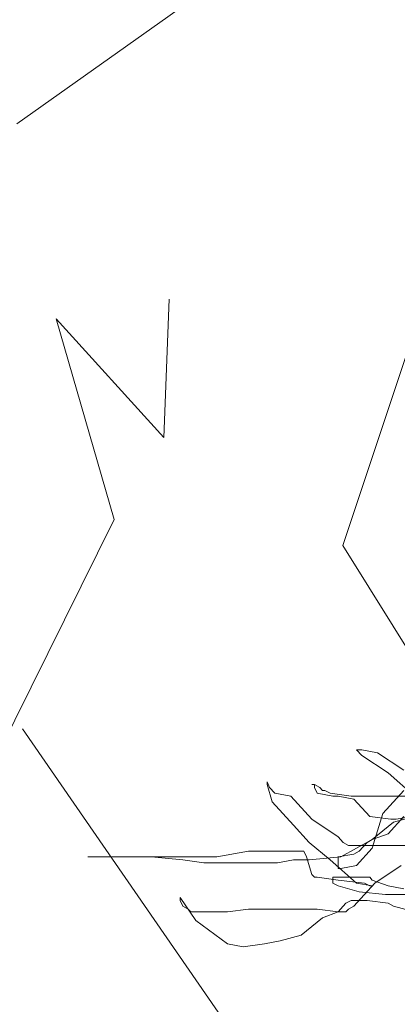
# Model space of a CAD drawing. Units: inches. Extents: x 1994 to 3075, y 3517 to 3950.
# Tile 37 of 58: x 1994.63804 to 1994.64257, y 3553.7375 to 3553.74931. Entities that reach past the tile are written whole.
import ezdxf

# ---------------------------------------------------------------- set-up
doc = ezdxf.new("R2010")
doc.units = ezdxf.units.IN
doc.layers.add('A-FURN-REFR', color=8, linetype='Continuous', lineweight=13)

msp = doc.modelspace()

# ---------------------------------------------------------------- linework, layer by layer
at = {"layer": 'A-FURN-REFR'}
for p, q in [((1994.638001, 3553.748064), (1994.640431, 3553.749786)), ((1994.639829, 3553.74596), (1994.639767, 3553.744298)), ((1994.642854, 3553.745822), (1994.641915, 3553.743002)), ((1994.638475, 3553.745722), (1994.639169, 3553.743315)), ((1994.639767, 3553.744298), (1994.638475, 3553.745722)), ((1994.639169, 3553.743315), (1994.637273, 3553.739491)), ((1994.641915, 3553.743002), (1994.643008, 3553.74125)), ((1994.638071, 3553.740802), (1994.641011, 3553.736552)), ((1994.642081, 3553.740552), (1994.642144, 3553.740552)), ((1994.642144, 3553.740482), (1994.642081, 3553.740552)), ((1994.642144, 3553.740552), (1994.642333, 3553.740517)), ((1994.64246, 3553.740274), (1994.642144, 3553.740482)), ((1994.642333, 3553.740517), (1994.642649, 3553.740308)), ((1994.642776, 3553.739996), (1994.64246, 3553.740274)), ((1994.641006, 3553.740169), (1994.641037, 3553.7401)), ((1994.641006, 3553.740135), (1994.641006, 3553.740169)), ((1994.641069, 3553.739926), (1994.641006, 3553.740135)), ((1994.641037, 3553.7401), (1994.641101, 3553.74003)), ((1994.641543, 3553.740135), (1994.641575, 3553.740135)), ((1994.641575, 3553.740135), (1994.641543, 3553.740135)), ((1994.641575, 3553.740135), (1994.641638, 3553.7401)), ((1994.641575, 3553.7401), (1994.641575, 3553.740135)), ((1994.641606, 3553.74003), (1994.641575, 3553.7401)), ((1994.641638, 3553.7401), (1994.64167, 3553.740065)), ((1994.641101, 3553.74003), (1994.64129, 3553.739996)), ((1994.64129, 3553.739996), (1994.641543, 3553.739718)), ((1994.641796, 3553.739996), (1994.641606, 3553.74003)), ((1994.64167, 3553.740065), (1994.641701, 3553.740065)), ((1994.641701, 3553.740065), (1994.641764, 3553.74003)), ((1994.641764, 3553.74003), (1994.642017, 3553.739996)), ((1994.641859, 3553.739996), (1994.641796, 3553.739996)), ((1994.642049, 3553.739961), (1994.641859, 3553.739996)), ((1994.642017, 3553.739996), (1994.643092, 3553.739996)), ((1994.642397, 3553.739787), (1994.642649, 3553.740065)), ((1994.641322, 3553.739648), (1994.641069, 3553.739926)), ((1994.642239, 3553.739752), (1994.642049, 3553.739961)), ((1994.642491, 3553.739718), (1994.642239, 3553.739752)), ((1994.642333, 3553.739579), (1994.642397, 3553.739787)), ((1994.642649, 3553.739752), (1994.64246, 3553.739544)), ((1994.642776, 3553.739752), (1994.642523, 3553.739683)), ((1994.642744, 3553.739752), (1994.642555, 3553.739718)), ((1994.641512, 3553.73944), (1994.641322, 3553.739648)), ((1994.641543, 3553.739718), (1994.641859, 3553.739509)), ((1994.642523, 3553.739683), (1994.64227, 3553.739474)), ((1994.642555, 3553.739718), (1994.642491, 3553.739718)), ((1994.641859, 3553.739509), (1994.641922, 3553.73944)), ((1994.64227, 3553.73937), (1994.642333, 3553.739579)), ((1994.64246, 3553.739544), (1994.64227, 3553.739474)), ((1994.641764, 3553.739231), (1994.641512, 3553.73944)), ((1994.64227, 3553.739474), (1994.641891, 3553.739266)), ((1994.641922, 3553.73944), (1994.641986, 3553.739405)), ((1994.641986, 3553.739405), (1994.643124, 3553.739405)), ((1994.642207, 3553.73944), (1994.642112, 3553.739335)), ((1994.64227, 3553.739474), (1994.642207, 3553.73944)), ((1994.638856, 3553.739266), (1994.640405, 3553.739266)), ((1994.639615, 3553.739266), (1994.638856, 3553.739266)), ((1994.639994, 3553.739231), (1994.639615, 3553.739266)), ((1994.640405, 3553.739266), (1994.640785, 3553.739335)), ((1994.640785, 3553.739335), (1994.641448, 3553.739335)), ((1994.641448, 3553.739335), (1994.64148, 3553.739266)), ((1994.64148, 3553.739266), (1994.641543, 3553.739057)), ((1994.641891, 3553.739266), (1994.641512, 3553.739231)), ((1994.642049, 3553.739301), (1994.641859, 3553.739266)), ((1994.641859, 3553.739266), (1994.641859, 3553.739127)), ((1994.642112, 3553.739335), (1994.642049, 3553.739301)), ((1994.642081, 3553.739162), (1994.64227, 3553.73937)), ((1994.640247, 3553.739196), (1994.639994, 3553.739231)), ((1994.641132, 3553.739196), (1994.640247, 3553.739196)), ((1994.641322, 3553.739231), (1994.641132, 3553.739196)), ((1994.641512, 3553.739231), (1994.641322, 3553.739231)), ((1994.642081, 3553.738953), (1994.641764, 3553.739231)), ((1994.641891, 3553.739127), (1994.642081, 3553.739162)), ((1994.642618, 3553.739162), (1994.642302, 3553.738953)), ((1994.641543, 3553.739057), (1994.641575, 3553.739023)), ((1994.641575, 3553.739023), (1994.641606, 3553.739023)), ((1994.641606, 3553.739023), (1994.641859, 3553.738988)), ((1994.641796, 3553.739023), (1994.641796, 3553.738953)), ((1994.642239, 3553.739023), (1994.641796, 3553.739023)), ((1994.641859, 3553.739127), (1994.641891, 3553.739127)), ((1994.64227, 3553.738988), (1994.642239, 3553.739023)), ((1994.641796, 3553.738953), (1994.641859, 3553.738918)), ((1994.641859, 3553.738988), (1994.642175, 3553.738953)), ((1994.641859, 3553.738918), (1994.642112, 3553.738849)), ((1994.642302, 3553.738953), (1994.642049, 3553.738675)), ((1994.64227, 3553.738918), (1994.642081, 3553.738953)), ((1994.642175, 3553.738953), (1994.642239, 3553.738918)), ((1994.642239, 3553.738918), (1994.64227, 3553.738918)), ((1994.64246, 3553.738918), (1994.64227, 3553.738988)), ((1994.642649, 3553.738884), (1994.64246, 3553.738918)), ((1994.642112, 3553.738849), (1994.642428, 3553.738814)), ((1994.642428, 3553.738814), (1994.642808, 3553.738814)), ((1994.639963, 3553.73878), (1994.640152, 3553.738502)), ((1994.639963, 3553.738745), (1994.639963, 3553.73878)), ((1994.639994, 3553.738675), (1994.639963, 3553.738745)), ((1994.640057, 3553.73864), (1994.639994, 3553.738675)), ((1994.641859, 3553.738606), (1994.641922, 3553.738675)), ((1994.641922, 3553.738675), (1994.641954, 3553.73871)), ((1994.641954, 3553.73871), (1994.642017, 3553.738745)), ((1994.642049, 3553.738675), (1994.641986, 3553.73864)), ((1994.642017, 3553.738745), (1994.642207, 3553.738745)), ((1994.642207, 3553.738745), (1994.64246, 3553.73871)), ((1994.64246, 3553.73871), (1994.642523, 3553.738675)), ((1994.642523, 3553.738675), (1994.642776, 3553.738606)), ((1994.640089, 3553.738606), (1994.640057, 3553.73864)), ((1994.640532, 3553.738606), (1994.640089, 3553.738606)), ((1994.640785, 3553.73864), (1994.640532, 3553.738606)), ((1994.641606, 3553.73864), (1994.640785, 3553.73864)), ((1994.641859, 3553.738606), (1994.641606, 3553.73864)), ((1994.64167, 3553.738536), (1994.641859, 3553.738606)), ((1994.641954, 3553.738606), (1994.641859, 3553.738606)), ((1994.641986, 3553.73864), (1994.641954, 3553.738606)), ((1994.640152, 3553.738502), (1994.640532, 3553.738224)), ((1994.641417, 3553.738328), (1994.64167, 3553.738536)), ((1994.641164, 3553.738258), (1994.641417, 3553.738328)), ((1994.640532, 3553.738224), (1994.640721, 3553.738189)), ((1994.640721, 3553.738189), (1994.640974, 3553.738224)), ((1994.640974, 3553.738224), (1994.641164, 3553.738258))]:
    msp.add_line(p, q, dxfattribs=at)

doc.saveas('drawing.dxf')
